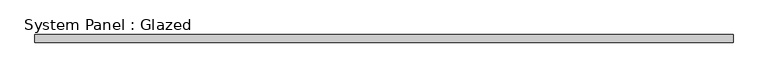
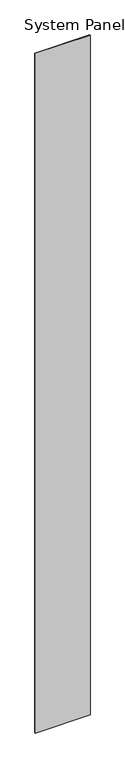
"""IFC4 building model written with IfcOpenShell, lengths in millimetres: plate geometry, System Panel : Glazed."""

from ifc_helpers import new_model, si_unit, origin, origin_with_axes, place, context, project, spatial, polyline, outline, extrude, source, transform, mapped, element, save


def system_panel_glazed_8ddfe979(model_context):
    return source(origin(), model_context, "Body", "SweptSolid", [
        extrude(outline(polyline([(1111.25, 19.05), (-1111.25, 19.05), (-1111.25, 44.45), (1111.25, 44.45), (1111.25, 19.05)])), origin_with_axes(), (0.0, 0.0, 1.0), 29133.8),
    ])


if __name__ == "__main__":
    model = new_model("IFC4")
    model_context = context("Model", 3, world=origin())
    ifc_project = project(units=[si_unit("LENGTHUNIT", "METRE", prefix="MILLI")], contexts=[model_context])
    site = spatial("IfcSite", under=ifc_project)
    building = spatial("IfcBuilding", under=site)
    placement = place(None, origin())
    system_panel_glazed_shape = system_panel_glazed_8ddfe979(model_context)
    element("IfcPlate", 1, ObjectType="System Panel : Glazed", at=placement, inside=building, context=model_context, shape_type="MappedRepresentation", body=[
        mapped(system_panel_glazed_shape, transform((0.0, 0.0, 0.0), x_axis=(1.0, 0.0, 0.0), y_axis=(0.0, 1.0, 0.0), z_axis=(0.0, 0.0, 1.0))),
    ])
    save(model, "model.ifc")

# Revit data of these elements
# Type "System Panel : Glazed"
#   Construction Type Id = "GSP4R"
#   Analytic Construction = "1/8 in Pilkington single glazing"
#   Visual Light Transmittance = 0.9
#   Solar Heat Gain Coefficient = 0.86
#   Heat Transfer Coefficient (U) = 1.18115 BTU/(h·ft²·°F)
# Element 1 (IfcPlate, "System Panel : Glazed")
#   Materials on its faces: "Glass"
# Materials
#   "Glass": class "Glass", colour RGB 0 128 192, transparency 0.75, Description = "Soda Lime Glass", Cost = 0
